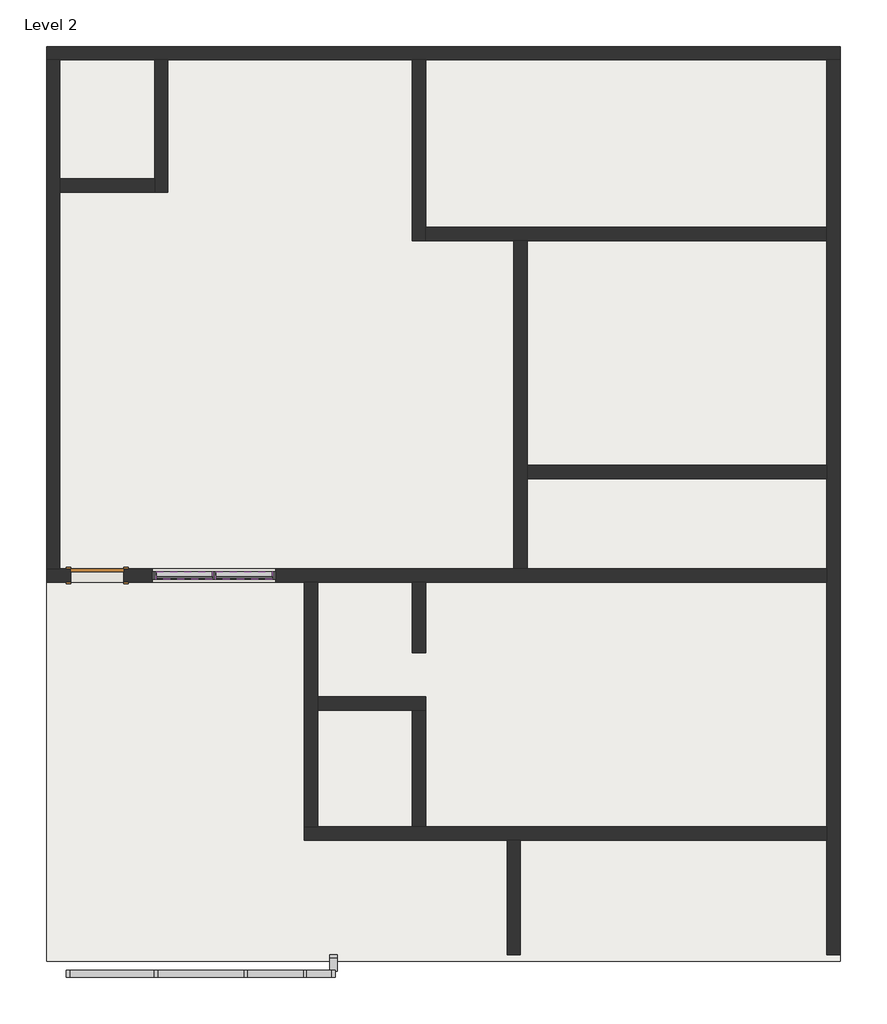
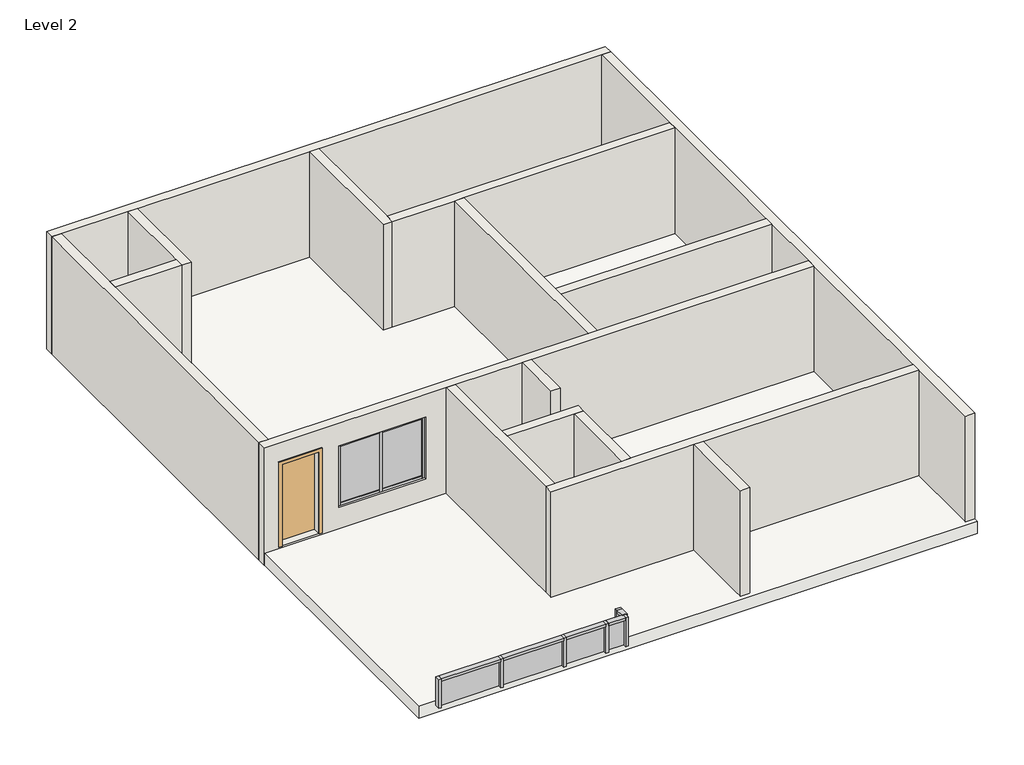
# One storey: 18 members, 16 walls, 7 plates, 1 door, 1 roof.
"""IFC4 building model written with IfcOpenShell, lengths in millimetres."""

from ifc_helpers import new_model, si_unit, frame, origin, place, context, project, spatial, polyline, outline, extrude, faceted_brep, transform, mapped, element, save
from components import door_a90ba1ad, member_801a2072, member_5210a67a, member_3f35b8d2, member_c8dfd0df, member_a139046c, member_b2e19614, member_b964ebf8, member_43d3509f, member_b2da0656, member_d8da5bea, member_29a45e76, system_panel_glazed_f5da27a7, system_panel_glazed_c279dccd, system_panel_glazed_038bf5f5, system_panel_glazed_a4f4dc30, system_panel_glazed_5fd0c891, system_panel_glazed_0590c333

model = new_model("IFC4")

# Units and contexts
model_context = context("Model", 3, world=origin())
ifc_project = project(units=[si_unit("LENGTHUNIT", "METRE", prefix="MILLI")], contexts=[model_context])

# Site, building, storey
site = spatial("IfcSite", under=ifc_project)
building = spatial("IfcBuilding", under=site)
storey = spatial("IfcBuildingStorey", under=building, Name="Level 2", Elevation=3048.0)

# Door
placement = place(None, origin())
door_shape = door_a90ba1ad(model_context)
element("IfcDoor", 1, ObjectType="Single-Flush : 36\" x 84\"", at=placement, inside=storey, context=model_context, shape_type="MappedRepresentation", body=[
    mapped(door_shape, transform((-17052.7047537, -14441.5428796, 3403.6), x_axis=(-1.0, 0.0, 0.0), y_axis=(0.0, -1.0, 0.0), z_axis=(0.0, 0.0, 1.0))),
])

# Members
member_shape = member_801a2072(model_context)
element("IfcMember", 2, ObjectType="Rectangular Mullion : 2.5\" x 5\" rectangular", at=placement, inside=storey, context=model_context, shape_type="MappedRepresentation", body=[
    mapped(member_shape, transform((-15001.6547537, -14441.5428796, 5504.9669794), x_axis=(0.0, 0.0, 1.0), y_axis=(0.0, 1.0, 0.0), z_axis=(-1.0, 0.0, 0.0))),
])
element("IfcMember", 3, ObjectType="Rectangular Mullion : 2.5\" x 5\" rectangular", at=placement, inside=storey, context=model_context, shape_type="MappedRepresentation", body=[
    mapped(member_shape, transform((-16036.7047537, -14441.5428796, 5504.9669794), x_axis=(0.0, 0.0, 1.0), y_axis=(0.0, 1.0, 0.0), z_axis=(-1.0, 0.0, 0.0))),
])
member_2_shape = member_5210a67a(model_context)
element("IfcMember", 4, ObjectType="Rectangular Mullion : 2.5\" x 5\" rectangular", at=placement, inside=storey, context=model_context, shape_type="MappedRepresentation", body=[
    mapped(member_2_shape, transform((-15033.4047537, -14441.5428796, 3904.8204327), x_axis=(-1.0, 0.0, 0.0), y_axis=(0.0, 1.0, 0.0), z_axis=(0.0, 0.0, -1.0))),
])
element("IfcMember", 5, ObjectType="Rectangular Mullion : 2.5\" x 5\" rectangular", at=placement, inside=storey, context=model_context, shape_type="MappedRepresentation", body=[
    mapped(member_shape, transform((-15065.1547537, -14441.5428796, 3904.8204327), x_axis=(0.0, 0.0, -1.0), y_axis=(0.0, 1.0, 0.0), z_axis=(1.0, 0.0, 0.0))),
])
element("IfcMember", 6, ObjectType="Rectangular Mullion : 2.5\" x 5\" rectangular", at=placement, inside=storey, context=model_context, shape_type="MappedRepresentation", body=[
    mapped(member_shape, transform((-14030.1047537, -14441.5428796, 3904.8204327), x_axis=(0.0, 0.0, -1.0), y_axis=(0.0, 1.0, 0.0), z_axis=(1.0, 0.0, 0.0))),
])
member_3_shape = member_3f35b8d2(model_context)
element("IfcMember", 7, ObjectType="Rectangular Mullion : 2.5\" x 5\" rectangular", at=placement, inside=storey, context=model_context, shape_type="MappedRepresentation", body=[
    mapped(member_3_shape, transform((-13966.6047537, -14441.5428796, 5504.9669794), x_axis=(1.0, 0.0, 0.0), y_axis=(0.0, 1.0, 0.0), z_axis=(0.0, 0.0, 1.0))),
])
element("IfcMember", 8, ObjectType="Rectangular Mullion : 2.5\" x 5\" rectangular", at=placement, inside=storey, context=model_context, shape_type="MappedRepresentation", body=[
    mapped(member_3_shape, transform((-16100.2047537, -14441.5428796, 3904.8204327), x_axis=(-1.0, 0.0, 0.0), y_axis=(0.0, 1.0, 0.0), z_axis=(0.0, 0.0, -1.0))),
])
member_4_shape = member_c8dfd0df(model_context)
element("IfcMember", 9, ObjectType="Rectangular Mullion : 2.5\" x 5\" rectangular", at=placement, inside=storey, context=model_context, shape_type="MappedRepresentation", body=[
    mapped(member_4_shape, transform((-17590.555135, -21324.9428796, 4101.2785678), x_axis=(-1.0, 0.0, 0.0), y_axis=(0.0, -1.0, 0.0), z_axis=(0.0, 0.0, 1.0))),
])
member_5_shape = member_a139046c(model_context)
element("IfcMember", 10, ObjectType="Rectangular Mullion : 2.5\" x 5\" rectangular", at=placement, inside=storey, context=model_context, shape_type="MappedRepresentation", body=[
    mapped(member_5_shape, transform((-16072.905135, -21324.9428796, 4101.2785678), x_axis=(0.0, 0.0, 1.0), y_axis=(0.0, -1.0, 0.0), z_axis=(1.0, 0.0, 0.0))),
])
member_6_shape = member_b2e19614(model_context)
element("IfcMember", 11, ObjectType="Rectangular Mullion : 2.5\" x 5\" rectangular", at=placement, inside=storey, context=model_context, shape_type="MappedRepresentation", body=[
    mapped(member_6_shape, transform((-16041.155135, -21324.9428796, 3352.8), x_axis=(1.0, 0.0, 0.0), y_axis=(0.0, -1.0, 0.0), z_axis=(0.0, 0.0, -1.0))),
])
element("IfcMember", 12, ObjectType="Rectangular Mullion : 2.5\" x 5\" rectangular", at=placement, inside=storey, context=model_context, shape_type="MappedRepresentation", body=[
    mapped(member_6_shape, transform((-14491.755135, -21324.9428796, 3352.8), x_axis=(1.0, 0.0, 0.0), y_axis=(0.0, -1.0, 0.0), z_axis=(0.0, 0.0, -1.0))),
])
element("IfcMember", 13, ObjectType="Rectangular Mullion : 2.5\" x 5\" rectangular", at=placement, inside=storey, context=model_context, shape_type="MappedRepresentation", body=[
    mapped(member_6_shape, transform((-13458.8218016, -21324.9428796, 3352.8), x_axis=(1.0, 0.0, 0.0), y_axis=(0.0, -1.0, 0.0), z_axis=(0.0, 0.0, -1.0))),
])
member_7_shape = member_b964ebf8(model_context)
element("IfcMember", 14, ObjectType="Rectangular Mullion : 2.5\" x 5\" rectangular", at=placement, inside=storey, context=model_context, shape_type="MappedRepresentation", body=[
    mapped(member_7_shape, transform((-14523.505135, -21324.9428796, 4101.2785678), x_axis=(0.0, 0.0, 1.0), y_axis=(0.0, -1.0, 0.0), z_axis=(1.0, 0.0, 0.0))),
])
member_8_shape = member_43d3509f(model_context)
element("IfcMember", 15, ObjectType="Rectangular Mullion : 2.5\" x 5\" rectangular", at=placement, inside=storey, context=model_context, shape_type="MappedRepresentation", body=[
    mapped(member_8_shape, transform((-13490.5718016, -21324.9428796, 4101.2785678), x_axis=(0.0, 0.0, 1.0), y_axis=(0.0, -1.0, 0.0), z_axis=(1.0, 0.0, 0.0))),
])
member_9_shape = member_b2da0656(model_context)
element("IfcMember", 16, ObjectType="Rectangular Mullion : 2.5\" x 5\" rectangular", at=placement, inside=storey, context=model_context, shape_type="MappedRepresentation", body=[
    mapped(member_9_shape, transform((-13005.855135, -21324.9428796, 4101.2785678), x_axis=(0.0, 0.0, 1.0), y_axis=(0.0, -1.0, 0.0), z_axis=(1.0, 0.0, 0.0))),
])
element("IfcMember", 17, ObjectType="Rectangular Mullion : 2.5\" x 5\" rectangular", at=placement, inside=storey, context=model_context, shape_type="MappedRepresentation", body=[
    mapped(member_4_shape, transform((-12942.355135, -21324.9428796, 3352.8), x_axis=(1.0, 0.0, 0.0), y_axis=(0.0, -1.0, 0.0), z_axis=(0.0, 0.0, -1.0))),
])
member_10_shape = member_d8da5bea(model_context)
element("IfcMember", 18, ObjectType="Rectangular Mullion : 2.5\" x 5\" rectangular", at=placement, inside=storey, context=model_context, shape_type="MappedRepresentation", body=[
    mapped(member_10_shape, transform((-12967.755135, -21280.4928796, 4101.2785678), x_axis=(0.0, 0.0, 1.0), y_axis=(-1.0, 0.0, 0.0), z_axis=(0.0, -1.0, 0.0))),
])
member_11_shape = member_29a45e76(model_context)
element("IfcMember", 19, ObjectType="Rectangular Mullion : 2.5\" x 5\" rectangular", at=placement, inside=storey, context=model_context, shape_type="MappedRepresentation", body=[
    mapped(member_11_shape, transform((-12967.755135, -20994.7428796, 4101.2785678), x_axis=(0.0, 1.0, 0.0), y_axis=(-1.0, 0.0, 0.0), z_axis=(0.0, 0.0, 1.0))),
])

# Plates
system_panel_glazed_shape = system_panel_glazed_f5da27a7(model_context)
element("IfcPlate", 20, ObjectType="System Panel : Glazed", at=placement, inside=storey, context=model_context, shape_type="MappedRepresentation", body=[
    mapped(system_panel_glazed_shape, transform((-14515.8797537, -14441.5428796, 3968.3204327), x_axis=(-1.0, 0.0, 0.0), y_axis=(0.0, -1.0, 0.0), z_axis=(0.0, 0.0, 1.0))),
])
element("IfcPlate", 21, ObjectType="System Panel : Glazed", at=placement, inside=storey, context=model_context, shape_type="MappedRepresentation", body=[
    mapped(system_panel_glazed_shape, transform((-15550.9297537, -14441.5428796, 3968.3204327), x_axis=(-1.0, 0.0, 0.0), y_axis=(0.0, -1.0, 0.0), z_axis=(0.0, 0.0, 1.0))),
])
system_panel_glazed_2_shape = system_panel_glazed_c279dccd(model_context)
element("IfcPlate", 22, ObjectType="System Panel : Glazed", at=placement, inside=storey, context=model_context, shape_type="MappedRepresentation", body=[
    mapped(system_panel_glazed_2_shape, transform((-16799.980135, -21324.9428796, 3352.8), x_axis=(1.0, 0.0, 0.0), y_axis=(0.0, 1.0, 0.0), z_axis=(0.0, 0.0, 1.0))),
])
system_panel_glazed_3_shape = system_panel_glazed_038bf5f5(model_context)
element("IfcPlate", 23, ObjectType="System Panel : Glazed", at=placement, inside=storey, context=model_context, shape_type="MappedRepresentation", body=[
    mapped(system_panel_glazed_3_shape, transform((-15266.455135, -21324.9428796, 3352.8), x_axis=(1.0, 0.0, 0.0), y_axis=(0.0, 1.0, 0.0), z_axis=(0.0, 0.0, 1.0))),
])
system_panel_glazed_4_shape = system_panel_glazed_a4f4dc30(model_context)
element("IfcPlate", 24, ObjectType="System Panel : Glazed", at=placement, inside=storey, context=model_context, shape_type="MappedRepresentation", body=[
    mapped(system_panel_glazed_4_shape, transform((-13975.2884683, -21324.9428796, 3352.8), x_axis=(1.0, 0.0, 0.0), y_axis=(0.0, 1.0, 0.0), z_axis=(0.0, 0.0, 1.0))),
])
system_panel_glazed_5_shape = system_panel_glazed_5fd0c891(model_context)
element("IfcPlate", 25, ObjectType="System Panel : Glazed", at=placement, inside=storey, context=model_context, shape_type="MappedRepresentation", body=[
    mapped(system_panel_glazed_5_shape, transform((-13216.4634683, -21324.9428796, 3352.8), x_axis=(1.0, 0.0, 0.0), y_axis=(0.0, 1.0, 0.0), z_axis=(0.0, 0.0, 1.0))),
])
system_panel_glazed_6_shape = system_panel_glazed_0590c333(model_context)
element("IfcPlate", 26, ObjectType="System Panel : Glazed", at=placement, inside=storey, context=model_context, shape_type="MappedRepresentation", body=[
    mapped(system_panel_glazed_6_shape, transform((-12967.755135, -21169.3678796, 3333.2738831), x_axis=(0.0, -1.0, 0.0), y_axis=(1.0, 0.0, 0.0), z_axis=(0.0, 0.0, 1.0))),
])

# Roof
element("IfcRoof", 27, ObjectType="Generic - 12\"", at=placement, inside=storey, context=model_context, shape_type="SweptSolid", body=[
    extrude(outline(polyline([(-17929.0047537, -5297.5428796), (-4213.0047537, -5297.5428796), (-4213.0047537, -21109.0428796), (-17929.0047537, -21109.0428796), (-17929.0047537, -5297.5428796)])), frame((0.0, 0.0, 3048.0), z_axis=(0.0, 0.0, 1.0), x_axis=(1.0, 0.0, 0.0)), (0.0, 0.0, 1.0), 304.8),
])

# Walls
element("IfcWall", 28, ObjectType="9\"", at=placement, inside=storey, context=model_context, shape_type="Brep", body=[
    faceted_brep([(-17929.0047537, -5526.1428796, 3048.0), (-17700.4047537, -5526.1428796, 3048.0), (-16062.1047537, -5526.1428796, 3048.0), (-15833.5047537, -5526.1428796, 3048.0), (-11604.4047537, -5526.1428796, 3048.0), (-11375.8047537, -5526.1428796, 3048.0), (-4441.6047537, -5526.1428796, 3048.0), (-4213.0047537, -5526.1428796, 3048.0), (-4213.0047537, -5526.1428796, 6096.0), (-4441.6047537, -5526.1428796, 6096.0), (-11375.8047537, -5526.1428796, 6096.0), (-11604.4047537, -5526.1428796, 6096.0), (-15833.5047537, -5526.1428796, 6096.0), (-16062.1047537, -5526.1428796, 6096.0), (-17700.4047537, -5526.1428796, 6096.0), (-17929.0047537, -5526.1428796, 6096.0), (-17929.0047537, -5297.5428796, 3048.0), (-17929.0047537, -5297.5428796, 6096.0), (-4213.0047537, -5297.5428796, 6096.0), (-4213.0047537, -5297.5428796, 3048.0)], [[[0, 1, 2, 3, 4, 5, 6, 7, 8, 9, 10, 11, 12, 13, 14, 15]], [[16, 17, 18, 19]], [[7, 6, 5, 4, 3, 2, 1, 0, 16, 19]], [[15, 14, 13, 12, 11, 10, 9, 8, 18, 17]], [[8, 7, 19, 18]], [[0, 15, 17, 16]]]),
])
element("IfcWall", 29, ObjectType="9\"", at=placement, inside=storey, context=model_context, shape_type="Brep", body=[
    faceted_brep([(-4441.6047537, -5526.1428796, 3048.0), (-4441.6047537, -8421.7428796, 3048.0), (-4441.6047537, -8650.3428796, 3048.0), (-4441.6047537, -12536.5428796, 3048.0), (-4441.6047537, -12765.1428796, 3048.0), (-4441.6047537, -14327.2428796, 3048.0), (-4441.6047537, -14555.8428796, 3048.0), (-4441.6047537, -18784.9428796, 3048.0), (-4441.6047537, -19013.5428796, 3048.0), (-4441.6047537, -20994.7428796, 3048.0), (-4441.6047537, -20994.7428796, 6096.0), (-4441.6047537, -19013.5428796, 6096.0), (-4441.6047537, -18784.9428796, 6096.0), (-4441.6047537, -14555.8428796, 6096.0), (-4441.6047537, -14327.2428796, 6096.0), (-4441.6047537, -12765.1428796, 6096.0), (-4441.6047537, -12536.5428796, 6096.0), (-4441.6047537, -8650.3428796, 6096.0), (-4441.6047537, -8421.7428796, 6096.0), (-4441.6047537, -5526.1428796, 6096.0), (-4213.0047537, -5526.1428796, 3048.0), (-4213.0047537, -5526.1428796, 6096.0), (-4213.0047537, -20994.7428796, 6096.0), (-4213.0047537, -20994.7428796, 3048.0)], [[[0, 1, 2, 3, 4, 5, 6, 7, 8, 9, 10, 11, 12, 13, 14, 15, 16, 17, 18, 19]], [[20, 21, 22, 23]], [[9, 8, 7, 6, 5, 4, 3, 2, 1, 0, 20, 23]], [[10, 9, 23, 22]], [[19, 18, 17, 16, 15, 14, 13, 12, 11, 10, 22, 21]], [[0, 19, 21, 20]]]),
])
element("IfcWall", 30, ObjectType="9\"", at=placement, inside=storey, context=model_context, shape_type="SweptSolid", body=[
    extrude(outline(polyline([(-9737.5047537, -19013.5428796), (-9737.5047537, -20994.7428796), (-9966.1047537, -20994.7428796), (-9966.1047537, -19013.5428796), (-9737.5047537, -19013.5428796)])), frame((0.0, 0.0, 3048.0), z_axis=(0.0, 0.0, 1.0), x_axis=(1.0, 0.0, 0.0)), (0.0, 0.0, 1.0), 3048.0),
])
element("IfcWall", 31, ObjectType="9\"", at=placement, inside=storey, context=model_context, shape_type="Brep", body=[
    faceted_brep([(-4441.6047537, -18784.9428796, 3048.0), (-11375.8047537, -18784.9428796, 3048.0), (-11604.4047537, -18784.9428796, 3048.0), (-13242.7047537, -18784.9428796, 3048.0), (-13471.3047537, -18784.9428796, 3048.0), (-13471.3047537, -18784.9428796, 6096.0), (-13242.7047537, -18784.9428796, 6096.0), (-11604.4047537, -18784.9428796, 6096.0), (-11375.8047537, -18784.9428796, 6096.0), (-4441.6047537, -18784.9428796, 6096.0), (-4441.6047537, -19013.5428796, 3048.0), (-4441.6047537, -19013.5428796, 6096.0), (-9737.5047537, -19013.5428796, 6096.0), (-9966.1047537, -19013.5428796, 6096.0), (-13471.3047537, -19013.5428796, 6096.0), (-13471.3047537, -19013.5428796, 3048.0), (-9966.1047537, -19013.5428796, 3048.0), (-9737.5047537, -19013.5428796, 3048.0)], [[[0, 1, 2, 3, 4, 5, 6, 7, 8, 9]], [[10, 11, 12, 13, 14, 15, 16, 17]], [[4, 3, 2, 1, 0, 10, 17, 16, 15]], [[9, 8, 7, 6, 5, 14, 13, 12, 11]], [[5, 4, 15, 14]], [[0, 9, 11, 10]]]),
])
element("IfcWall", 32, ObjectType="9\"", at=placement, inside=storey, context=model_context, shape_type="Brep", body=[
    faceted_brep([(-13242.7047537, -18784.9428796, 3048.0), (-13242.7047537, -16765.6428796, 3048.0), (-13242.7047537, -16537.0428796, 3048.0), (-13242.7047537, -14555.8428796, 3048.0), (-13242.7047537, -14555.8428796, 6096.0), (-13242.7047537, -16537.0428796, 6096.0), (-13242.7047537, -16765.6428796, 6096.0), (-13242.7047537, -18784.9428796, 6096.0), (-13471.3047537, -18784.9428796, 3048.0), (-13471.3047537, -18784.9428796, 6096.0), (-13471.3047537, -14555.8428796, 6096.0), (-13471.3047537, -14555.8428796, 3048.0)], [[[0, 1, 2, 3, 4, 5, 6, 7]], [[8, 9, 10, 11]], [[3, 2, 1, 0, 8, 11]], [[7, 6, 5, 4, 10, 9]], [[0, 7, 9, 8]], [[4, 3, 11, 10]]]),
])
element("IfcWall", 33, ObjectType="9\"", at=placement, inside=storey, context=model_context, shape_type="Brep", body=[
    faceted_brep([(-4441.6047537, -14327.2428796, 3048.0), (-9623.2047537, -14327.2428796, 3048.0), (-9851.8047537, -14327.2428796, 3048.0), (-17700.4047537, -14327.2428796, 3048.0), (-17929.0047537, -14327.2428796, 3048.0), (-17929.0047537, -14327.2428796, 6096.0), (-17700.4047537, -14327.2428796, 6096.0), (-9851.8047537, -14327.2428796, 6096.0), (-9623.2047537, -14327.2428796, 6096.0), (-4441.6047537, -14327.2428796, 6096.0), (-17509.9047537, -14327.2428796, 3403.6), (-16595.5047537, -14327.2428796, 3403.6), (-16595.5047537, -14327.2428796, 5537.2), (-17509.9047537, -14327.2428796, 5537.2), (-13966.6047537, -14327.2428796, 3904.8204327), (-13966.6047537, -14327.2428796, 5504.9669794), (-16100.2047537, -14327.2428796, 5504.9669794), (-16100.2047537, -14327.2428796, 3904.8204327), (-17929.0047537, -14555.8428796, 3048.0), (-13471.3047537, -14555.8428796, 3048.0), (-13242.7047537, -14555.8428796, 3048.0), (-11604.4047537, -14555.8428796, 3048.0), (-11375.8047537, -14555.8428796, 3048.0), (-4441.6047537, -14555.8428796, 3048.0), (-4441.6047537, -14555.8428796, 6096.0), (-11375.8047537, -14555.8428796, 6096.0), (-11604.4047537, -14555.8428796, 6096.0), (-13242.7047537, -14555.8428796, 6096.0), (-13471.3047537, -14555.8428796, 6096.0), (-17929.0047537, -14555.8428796, 6096.0), (-16595.5047537, -14555.8428796, 3403.6), (-17509.9047537, -14555.8428796, 3403.6), (-17509.9047537, -14555.8428796, 5537.2), (-16595.5047537, -14555.8428796, 5537.2), (-13966.6047537, -14555.8428796, 5504.9669794), (-13966.6047537, -14555.8428796, 3904.8204327), (-16100.2047537, -14555.8428796, 3904.8204327), (-16100.2047537, -14555.8428796, 5504.9669794)], [[[0, 1, 2, 3, 4, 5, 6, 7, 8, 9], [10, 11, 12, 13], [14, 15, 16, 17]], [[18, 19, 20, 21, 22, 23, 24, 25, 26, 27, 28, 29], [30, 31, 32, 33], [34, 35, 36, 37]], [[4, 3, 2, 1, 0, 23, 22, 21, 20, 19, 18]], [[9, 8, 7, 6, 5, 29, 28, 27, 26, 25, 24]], [[5, 4, 18, 29]], [[0, 9, 24, 23]], [[31, 30, 11, 10]], [[32, 31, 10, 13]], [[33, 32, 13, 12]], [[30, 33, 12, 11]], [[14, 35, 34, 15]], [[15, 34, 37, 16]], [[16, 37, 36, 17]], [[35, 14, 17, 36]]]),
])
element("IfcWall", 34, ObjectType="9\"", at=placement, inside=storey, context=model_context, shape_type="Brep", body=[
    faceted_brep([(-17929.0047537, -5526.1428796, 3048.0), (-17929.0047537, -14327.2428796, 3048.0), (-17929.0047537, -14327.2428796, 6096.0), (-17929.0047537, -5526.1428796, 6096.0), (-17700.4047537, -5526.1428796, 3048.0), (-17700.4047537, -5526.1428796, 6096.0), (-17700.4047537, -7583.5428796, 6096.0), (-17700.4047537, -7812.1428796, 6096.0), (-17700.4047537, -14327.2428796, 6096.0), (-17700.4047537, -14327.2428796, 3048.0), (-17700.4047537, -7812.1428796, 3048.0), (-17700.4047537, -7583.5428796, 3048.0)], [[[0, 1, 2, 3]], [[4, 5, 6, 7, 8, 9, 10, 11]], [[1, 0, 4, 11, 10, 9]], [[3, 2, 8, 7, 6, 5]], [[0, 3, 5, 4]], [[2, 1, 9, 8]]]),
])
element("IfcWall", 35, ObjectType="9\"", at=placement, inside=storey, context=model_context, shape_type="Brep", body=[
    faceted_brep([(-13242.7047537, -16765.6428796, 3048.0), (-11604.4047537, -16765.6428796, 3048.0), (-11375.8047537, -16765.6428796, 3048.0), (-11375.8047537, -16765.6428796, 6096.0), (-11604.4047537, -16765.6428796, 6096.0), (-13242.7047537, -16765.6428796, 6096.0), (-13242.7047537, -16537.0428796, 3048.0), (-13242.7047537, -16537.0428796, 6096.0), (-11375.8047537, -16537.0428796, 6096.0), (-11375.8047537, -16537.0428796, 3048.0)], [[[0, 1, 2, 3, 4, 5]], [[6, 7, 8, 9]], [[2, 1, 0, 6, 9]], [[5, 4, 3, 8, 7]], [[0, 5, 7, 6]], [[3, 2, 9, 8]]]),
])
element("IfcWall", 36, ObjectType="9\"", at=placement, inside=storey, context=model_context, shape_type="SweptSolid", body=[
    extrude(outline(polyline([(-11604.4047537, -18784.9428796), (-11604.4047537, -16765.6428796), (-11375.8047537, -16765.6428796), (-11375.8047537, -18784.9428796), (-11604.4047537, -18784.9428796)])), frame((0.0, 0.0, 3048.0), z_axis=(0.0, 0.0, 1.0), x_axis=(1.0, 0.0, 0.0)), (0.0, 0.0, 1.0), 3048.0),
])
element("IfcWall", 37, ObjectType="9\"", at=placement, inside=storey, context=model_context, shape_type="Brep", body=[
    faceted_brep([(-9623.2047537, -14327.2428796, 3048.0), (-9623.2047537, -12765.1428796, 3048.0), (-9623.2047537, -12536.5428796, 3048.0), (-9623.2047537, -8650.3428796, 3048.0), (-9623.2047537, -8650.3428796, 6096.0), (-9623.2047537, -12536.5428796, 6096.0), (-9623.2047537, -12765.1428796, 6096.0), (-9623.2047537, -14327.2428796, 6096.0), (-9851.8047537, -14327.2428796, 3048.0), (-9851.8047537, -14327.2428796, 6096.0), (-9851.8047537, -8650.3428796, 6096.0), (-9851.8047537, -8650.3428796, 3048.0)], [[[0, 1, 2, 3, 4, 5, 6, 7]], [[8, 9, 10, 11]], [[3, 2, 1, 0, 8, 11]], [[7, 6, 5, 4, 10, 9]], [[0, 7, 9, 8]], [[4, 3, 11, 10]]]),
])
element("IfcWall", 38, ObjectType="9\"", at=placement, inside=storey, context=model_context, shape_type="Brep", body=[
    faceted_brep([(-11375.8047537, -8650.3428796, 3048.0), (-9851.8047537, -8650.3428796, 3048.0), (-9623.2047537, -8650.3428796, 3048.0), (-4441.6047537, -8650.3428796, 3048.0), (-4441.6047537, -8650.3428796, 6096.0), (-9623.2047537, -8650.3428796, 6096.0), (-9851.8047537, -8650.3428796, 6096.0), (-11375.8047537, -8650.3428796, 6096.0), (-11375.8047537, -8421.7428796, 3048.0), (-11375.8047537, -8421.7428796, 6096.0), (-4441.6047537, -8421.7428796, 6096.0), (-4441.6047537, -8421.7428796, 3048.0)], [[[0, 1, 2, 3, 4, 5, 6, 7]], [[8, 9, 10, 11]], [[3, 2, 1, 0, 8, 11]], [[7, 6, 5, 4, 10, 9]], [[4, 3, 11, 10]], [[0, 7, 9, 8]]]),
])
element("IfcWall", 39, ObjectType="9\"", at=placement, inside=storey, context=model_context, shape_type="Brep", body=[
    faceted_brep([(-11604.4047537, -5526.1428796, 3048.0), (-11604.4047537, -8650.3428796, 3048.0), (-11604.4047537, -8650.3428796, 6096.0), (-11604.4047537, -5526.1428796, 6096.0), (-11375.8047537, -5526.1428796, 3048.0), (-11375.8047537, -5526.1428796, 6096.0), (-11375.8047537, -8421.7428796, 6096.0), (-11375.8047537, -8650.3428796, 6096.0), (-11375.8047537, -8650.3428796, 3048.0), (-11375.8047537, -8421.7428796, 3048.0)], [[[0, 1, 2, 3]], [[4, 5, 6, 7, 8, 9]], [[1, 0, 4, 9, 8]], [[3, 2, 7, 6, 5]], [[0, 3, 5, 4]], [[2, 1, 8, 7]]]),
])
element("IfcWall", 40, ObjectType="9\"", at=placement, inside=storey, context=model_context, shape_type="Brep", body=[
    faceted_brep([(-16062.1047537, -5526.1428796, 3048.0), (-16062.1047537, -7583.5428796, 3048.0), (-16062.1047537, -7812.1428796, 3048.0), (-16062.1047537, -7812.1428796, 6096.0), (-16062.1047537, -7583.5428796, 6096.0), (-16062.1047537, -5526.1428796, 6096.0), (-15833.5047537, -5526.1428796, 3048.0), (-15833.5047537, -5526.1428796, 6096.0), (-15833.5047537, -7812.1428796, 6096.0), (-15833.5047537, -7812.1428796, 3048.0)], [[[0, 1, 2, 3, 4, 5]], [[6, 7, 8, 9]], [[2, 1, 0, 6, 9]], [[5, 4, 3, 8, 7]], [[0, 5, 7, 6]], [[3, 2, 9, 8]]]),
])
element("IfcWall", 41, ObjectType="9\"", at=placement, inside=storey, context=model_context, shape_type="SweptSolid", body=[
    extrude(outline(polyline([(-17700.4047537, -7583.5428796), (-16062.1047537, -7583.5428796), (-16062.1047537, -7812.1428796), (-17700.4047537, -7812.1428796), (-17700.4047537, -7583.5428796)])), frame((0.0, 0.0, 3048.0), z_axis=(0.0, 0.0, 1.0), x_axis=(1.0, 0.0, 0.0)), (0.0, 0.0, 1.0), 3048.0),
])
element("IfcWall", 42, ObjectType="9\"", at=placement, inside=storey, context=model_context, shape_type="SweptSolid", body=[
    extrude(outline(polyline([(-11604.4047537, -15775.0428796), (-11604.4047537, -14555.8428796), (-11375.8047537, -14555.8428796), (-11375.8047537, -15775.0428796), (-11604.4047537, -15775.0428796)])), frame((0.0, 0.0, 3048.0), z_axis=(0.0, 0.0, 1.0), x_axis=(1.0, 0.0, 0.0)), (0.0, 0.0, 1.0), 3048.0),
])
element("IfcWall", 43, ObjectType="9\"", at=placement, inside=storey, context=model_context, shape_type="SweptSolid", body=[
    extrude(outline(polyline([(-4441.6047537, -12765.1428796), (-9623.2047537, -12765.1428796), (-9623.2047537, -12536.5428796), (-4441.6047537, -12536.5428796), (-4441.6047537, -12765.1428796)])), frame((0.0, 0.0, 3048.0), z_axis=(0.0, 0.0, 1.0), x_axis=(1.0, 0.0, 0.0)), (0.0, 0.0, 1.0), 3048.0),
])

save(model, "model.ifc")

# Revit data of these elements
# Type "Single-Flush : 36\" x 84\""
#   Type Mark = "1"
#   Construction Type Id = "MDOOR"
#   Assembly Code = "C1020"
#   Analytic Construction = "Metal"
#   Thickness = 0' - 2"
#   Heat Transfer Coefficient (U) = 0.651978 BTU/(h·ft²·°F)
#   Height = 7' - 0"
#   Trim Projection Ext = 0' - 1"
#   Trim Projection Int = 0' - 1"
#   Trim Width = 0' - 3"
#   Width = 3' - 0"
#   Define Thermal Properties by = 1
#   Define Thermal Properties by = 1
#   Door Material = Door - Panel
#   Frame Material = Door - Frame
#   Visual Light Transmittance = 0
#   Solar Heat Gain Coefficient = 0
#   Function = (empty or 0)
#   Wall Closure = (empty or 0)
# Type "Rectangular Mullion : 2.5\" x 5\" rectangular"
#   built-in parameter 1007304 = 0.416667 (stored number, unit not read)
#   built-in parameter 1007301 = 0.104167 (stored number, unit not read)
#   built-in parameter 1007300 = 0.104167 (stored number, unit not read)
# Type "System Panel : Glazed"
#   Construction Type Id = "GSP4R"
#   Analytic Construction = "1/8 in Pilkington single glazing"
#   Visual Light Transmittance = 0.9
#   Solar Heat Gain Coefficient = 0.86
#   Heat Transfer Coefficient (U) = 1.18115 BTU/(h·ft²·°F)
#   Define Thermal Properties by = 1
# Type "Generic - 12\""
#   Assembly Code = "B1020"
#   Layers, outside or top first: 1' - 0" no material (function 1)
# Type "9\""
#   Assembly Code = "B2010"
#   Layers, outside or top first: 0' - 9" no material (function 1)
# Element 1 (IfcDoor, "Single-Flush : 36\" x 84\"")
#   Phase Created = New Construction
#   Materials on its faces: "Door - Frame", "Door - Panel"
# Elements 2, 3, 4, 5, 6, 7, 8, 9, 10, 11, 12, 13, 14, 15, 16, 17, 18, 19 (IfcMember, "Rectangular Mullion : 2.5\" x 5\" rectangular")
#   Phase Created = New Construction
#   Materials on its faces: "Aluminum"
# Elements 20, 21, 22, 23, 24, 25, 26 (IfcPlate, "System Panel : Glazed")
#   Phase Created = New Construction
#   Materials on its faces: "Glass"
# Element 27 (IfcRoof, "Generic - 12\"")
#   built-in parameter 1001705 = 11 (stored number, unit not read)
#   built-in parameter 1001710 = 33615
#   Phase Created = New Construction
#   Materials on its faces: "Default Roof"
# Elements 28, 29, 30, 31, 32, 33, 34, 35, 36, 37, 38, 39, 40, 41, 42, 43 (IfcWall, "9\"")
#   Top Offset = 0' - 0"
#   Base Offset = 0' - 0"
#   Unconnected Height = 10' - 0"
#   wall height = 10' - 0"
#   Phase Created = New Construction
#   Base Constraint = Level 2
#   Materials on its faces: "Default Wall"
# Materials
#   "Door - Panel": class "Wood", colour RGB 210 159 95, transparency 0, Cost = 0
#   "Door - Frame": colour RGB 118 70 51, transparency 0, Cost = 0
#   "Aluminum": class "Metal", colour RGB 247 247 247, transparency 0, Description = "Aluminum 6061", Cost = 0
#   "Glass": class "Glass", colour RGB 0 128 192, transparency 0.75, Description = "Soda Lime Glass", Cost = 0
#   "Default Roof": colour RGB 88 101 114, transparency 0, Cost = 0
#   "Default Wall": colour RGB 128 128 128, transparency 0, Cost = 0
